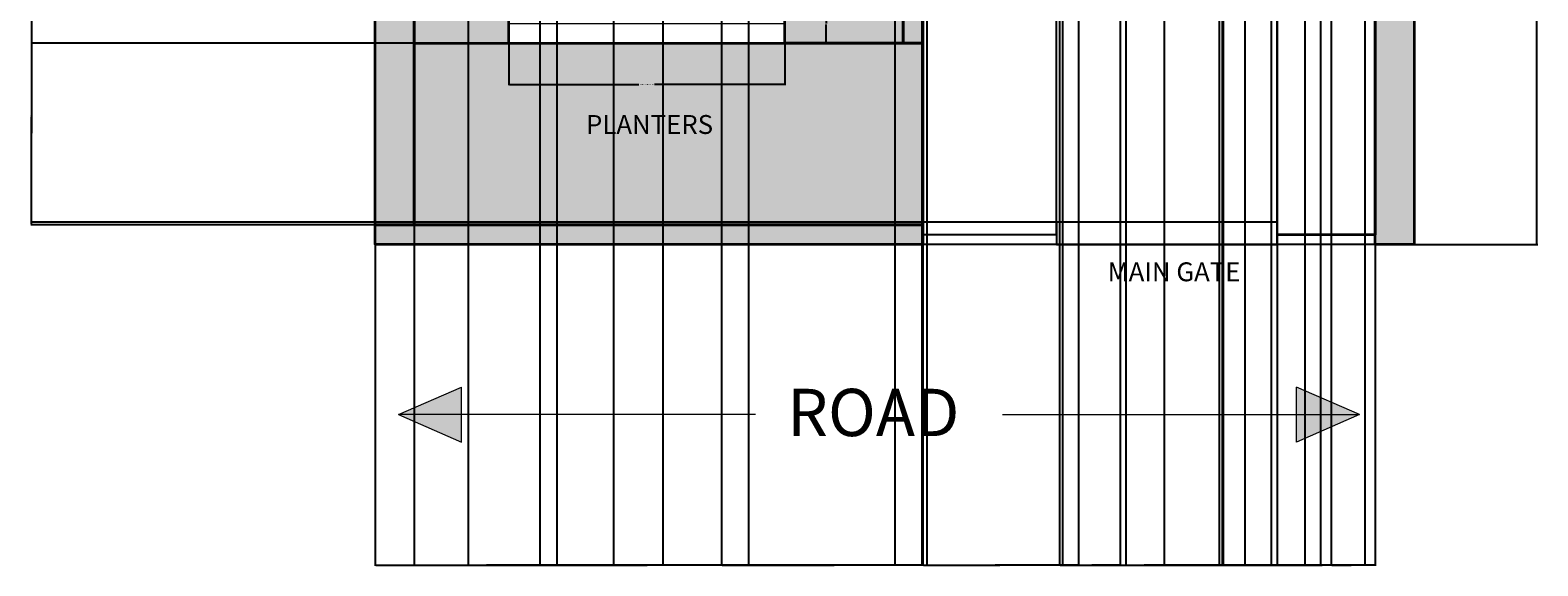
# Model space of a CAD drawing. Units: inches. Extents: x 2035 to 2384, y 1427 to 2020.
# Tile 1 of 7: x 2035 to 2383, y 1427 to 1551. Entities that reach past the tile are written whole.
import ezdxf

# ---------------------------------------------------------------- set-up
doc = ezdxf.new("R2010")
doc.units = ezdxf.units.IN
for name, color, linetype, lineweight in [('A-ANNO-DIMS', 2, 'Continuous', 18), ('A-ANNO-SYMB', 201, 'Continuous', 18), ('A-ANNO-TEXT', 201, 'Continuous', 18), ('A-SITE-GATE', 52, 'Continuous', 25), ('A-WALL-PATT', 140, 'Continuous', 13), ('C-PROP', 7, 'Continuous', 25), ('L-PLNT-PATT', 112, 'Continuous', 13), ('WALL', 140, 'Continuous', 35), ('WIN', 230, 'Continuous', 18)]:
    doc.layers.add(name, color=color, linetype=linetype, lineweight=lineweight)
doc.styles.get("Standard").update_dxf_attribs({"font": 'arial.ttf'})
doc.dimstyles.get("Standard").update_dxf_attribs({"dimtxt": 0.18, "dimasz": 0.18, "dimexe": 0.18, "dimexo": 0.0625, "dimgap": 0.09, "dimtad": 0, "dimtih": 1, "dimtoh": 1, "dimdec": 4, "dimzin": 0, "dimdsep": 46, "dimtxsty": 'Standard', "dimcen": 0.09, "dimadec": 0, "dimazin": 0, "dimtfac": 1, "dimtdec": 4, "dimtofl": 0, "dimtmove": 0, "dimatfit": 3, "dimfxl": 1, "dimtolj": 1, "dimtzin": 0, "dimarcsym": 0})

# ---------------------------------------------------------------- blocks, each defined once
blk = doc.blocks.new('WIN-BEDROOM')
blk.add_line((0, 4.5), (63.76, 4.5))
blk.add_lwpolyline([(0, 9), (63.76, 9), (63.76, 0), (0, 0)], close=True)
blk = doc.blocks.new('*D14')
at = {"layer": 'A-ANNO-DIMS', "color": 0, "lineweight": -2, "transparency": 16777216}
for p, q in [((2145.62, 1547.82), (2145.62, 1538.14)), ((2209.38, 1547.82), (2209.38, 1538.14)), ((2145.8, 1538.32), (2175.7, 1538.32)), ((2209.2, 1538.32), (2179.29, 1538.32))]:
    blk.add_line(p, q, dxfattribs=at)
at = {"layer": 'A-ANNO-DIMS', "color": 0, "lineweight": 100, "transparency": 16777216}
for points in [[(2145.8, 1538.35), (2145.8, 1538.29), (2145.62, 1538.32)], [(2209.2, 1538.35), (2209.2, 1538.29), (2209.38, 1538.32)]]:
    blk.add_solid(points, dxfattribs=at)
at = {"layer": 'Defpoints', "color": 0, "lineweight": 100, "transparency": 16777216}
for p in [(2145.62, 1547.88), (2209.38, 1547.88), (2209.38, 1538.32)]:
    blk.add_point(p, dxfattribs=at)
at = {"layer": 'A-ANNO-DIMS', "color": 0, "transparency": 16777216, "insert": (2177.5, 1538.32), "char_height": 0.18, "attachment_point": 5}
blk.add_mtext('\\A1;BEDROOM WINDOW 64 TYP.', dxfattribs=at)
blk = doc.blocks.new('*D15')
at = {"layer": 'A-ANNO-DIMS', "color": 0, "lineweight": -2, "transparency": 16777216}
for p, q in [((2209.44, 1556.88), (2219.12, 1556.88)), ((2218.94, 1556.7), (2218.94, 1552.56)), ((2218.94, 1548.06), (2218.94, 1552.2)), ((2209.44, 1547.88), (2219.12, 1547.88))]:
    blk.add_line(p, q, dxfattribs=at)
at = {"layer": 'A-ANNO-DIMS', "color": 0, "lineweight": 100, "transparency": 16777216}
for points in [[(2218.91, 1556.7), (2218.97, 1556.7), (2218.94, 1556.88)], [(2218.91, 1548.06), (2218.97, 1548.06), (2218.94, 1547.88)]]:
    blk.add_solid(points, dxfattribs=at)
at = {"layer": 'Defpoints', "color": 0, "lineweight": 100, "transparency": 16777216}
for p in [(2209.38, 1556.88), (2218.94, 1556.88), (2209.38, 1547.88)]:
    blk.add_point(p, dxfattribs=at)
at = {"layer": 'A-ANNO-DIMS', "color": 0, "transparency": 16777216, "insert": (2218.94, 1552.38), "char_height": 0.18, "attachment_point": 5}
blk.add_mtext('\\A1;9 TYP.', dxfattribs=at)
blk = doc.blocks.new('*D23')
at = {"layer": 'A-ANNO-DIMS', "color": 0, "lineweight": -2, "transparency": 16777216}
for p, q in [((2354.82, 1981.38), (2383.33, 1981.38)), ((2383.15, 1981.2), (2383.15, 1741.56)), ((2383.15, 1501.56), (2383.15, 1741.2)), ((2354.82, 1501.38), (2383.33, 1501.38))]:
    blk.add_line(p, q, dxfattribs=at)
at = {"layer": 'A-ANNO-DIMS', "color": 0, "lineweight": 100, "transparency": 16777216}
for points in [[(2383.12, 1981.2), (2383.18, 1981.2), (2383.15, 1981.38)], [(2383.12, 1501.56), (2383.18, 1501.56), (2383.15, 1501.38)]]:
    blk.add_solid(points, dxfattribs=at)
at = {"layer": 'Defpoints', "color": 0, "lineweight": 100, "transparency": 16777216}
for p in [(2354.75, 1981.38), (2383.15, 1981.38), (2354.75, 1501.38)]:
    blk.add_point(p, dxfattribs=at)
at = {"layer": 'A-ANNO-DIMS', "color": 0, "transparency": 16777216, "insert": (2383.15, 1741.38), "char_height": 0.18, "attachment_point": 5}
blk.add_mtext('\\A1;480', dxfattribs=at)
blk = doc.blocks.new('*D24')
at = {"layer": 'A-ANNO-DIMS', "color": 0, "lineweight": -2, "transparency": 16777216}
for p, q in [((2114.75, 1501.32), (2114.75, 1427.17)), ((2241.25, 1501.32), (2241.25, 1427.17)), ((2114.93, 1427.35), (2177.62, 1427.35)), ((2241.07, 1427.35), (2178.39, 1427.35))]:
    blk.add_line(p, q, dxfattribs=at)
at = {"layer": 'A-ANNO-DIMS', "color": 0, "lineweight": 100, "transparency": 16777216}
for points in [[(2114.93, 1427.38), (2114.93, 1427.32), (2114.75, 1427.35)], [(2241.07, 1427.38), (2241.07, 1427.32), (2241.25, 1427.35)]]:
    blk.add_solid(points, dxfattribs=at)
at = {"layer": 'Defpoints', "color": 0, "lineweight": 100, "transparency": 16777216}
for p in [(2114.75, 1501.38), (2241.25, 1501.38), (2241.25, 1427.35)]:
    blk.add_point(p, dxfattribs=at)
at = {"layer": 'A-ANNO-DIMS', "color": 0, "transparency": 16777216, "insert": (2178, 1427.35), "char_height": 0.18, "attachment_point": 5}
blk.add_mtext('\\A1;126.5', dxfattribs=at)
blk = doc.blocks.new('*D25')
at = {"layer": 'A-ANNO-DIMS', "color": 0, "lineweight": -2, "transparency": 16777216}
for p, q in [((2241.25, 1503.69), (2241.25, 2009.96)), ((2241.43, 2009.78), (2256.26, 2009.78)), ((2272.01, 2009.78), (2257.18, 2009.78)), ((2272.19, 1503.69), (2272.19, 2009.96))]:
    blk.add_line(p, q, dxfattribs=at)
at = {"layer": 'A-ANNO-DIMS', "color": 0, "lineweight": 100, "transparency": 16777216}
for points in [[(2241.43, 2009.81), (2241.43, 2009.75), (2241.25, 2009.78)], [(2272.01, 2009.81), (2272.01, 2009.75), (2272.19, 2009.78)]]:
    blk.add_solid(points, dxfattribs=at)
at = {"layer": 'Defpoints', "color": 0, "lineweight": 100, "transparency": 16777216}
for p in [(2272.19, 2009.78), (2241.25, 1503.63), (2272.19, 1503.63)]:
    blk.add_point(p, dxfattribs=at)
at = {"layer": 'A-ANNO-DIMS', "color": 0, "transparency": 16777216, "insert": (2256.72, 2009.78), "char_height": 0.18, "attachment_point": 5}
blk.add_mtext('\\A1;30.935', dxfattribs=at)
blk = doc.blocks.new('*D26')
at = {"layer": 'A-ANNO-DIMS', "color": 0, "lineweight": -2, "transparency": 16777216}
for p, q in [((2272.19, 1506.56), (2272.19, 2009.96)), ((2272.37, 2009.78), (2297.26, 2009.78)), ((2322.93, 2009.78), (2298.04, 2009.78)), ((2323.11, 1506.56), (2323.11, 2009.96))]:
    blk.add_line(p, q, dxfattribs=at)
at = {"layer": 'A-ANNO-DIMS', "color": 0, "lineweight": 100, "transparency": 16777216}
for points in [[(2272.37, 2009.81), (2272.37, 2009.75), (2272.19, 2009.78)], [(2322.93, 2009.81), (2322.93, 2009.75), (2323.11, 2009.78)]]:
    blk.add_solid(points, dxfattribs=at)
at = {"layer": 'Defpoints', "color": 0, "lineweight": 100, "transparency": 16777216}
for p in [(2323.11, 2009.78), (2272.19, 1506.5), (2323.11, 1506.5)]:
    blk.add_point(p, dxfattribs=at)
at = {"layer": 'A-ANNO-DIMS', "color": 0, "transparency": 16777216, "insert": (2297.65, 2009.78), "char_height": 0.18, "attachment_point": 5}
blk.add_mtext('\\A1;50.92', dxfattribs=at)
blk = doc.blocks.new('*D27')
at = {"layer": 'A-ANNO-DIMS', "color": 0, "lineweight": -2, "transparency": 16777216}
for p, q in [((2123.69, 1547.88), (2035.17, 1547.88)), ((2035.35, 1547.7), (2035.35, 1527.06)), ((2035.35, 1506.06), (2035.35, 1526.7)), ((2123.69, 1505.88), (2035.17, 1505.88))]:
    blk.add_line(p, q, dxfattribs=at)
at = {"layer": 'A-ANNO-DIMS', "color": 0, "lineweight": 100, "transparency": 16777216}
for points in [[(2035.32, 1547.7), (2035.38, 1547.7), (2035.35, 1547.88)], [(2035.32, 1506.06), (2035.38, 1506.06), (2035.35, 1505.88)]]:
    blk.add_solid(points, dxfattribs=at)
at = {"layer": 'Defpoints', "color": 0, "lineweight": 100, "transparency": 16777216}
for p in [(2035.35, 1547.88), (2123.75, 1547.88), (2123.75, 1505.88)]:
    blk.add_point(p, dxfattribs=at)
at = {"layer": 'A-ANNO-DIMS', "color": 0, "transparency": 16777216, "insert": (2035.35, 1526.88), "char_height": 0.18, "attachment_point": 5}
blk.add_mtext('\\A1;42', dxfattribs=at)
blk = doc.blocks.new('*D28')
at = {"layer": 'A-ANNO-DIMS', "color": 0, "lineweight": -2, "transparency": 16777216}
for p, q in [((2345.69, 1555.63), (2035.17, 1555.63)), ((2035.35, 1555.45), (2035.35, 1531.25)), ((2035.35, 1506.68), (2035.35, 1530.88)), ((2323.05, 1506.5), (2035.17, 1506.5))]:
    blk.add_line(p, q, dxfattribs=at)
at = {"layer": 'A-ANNO-DIMS', "color": 0, "lineweight": 100, "transparency": 16777216}
for points in [[(2035.32, 1555.45), (2035.38, 1555.45), (2035.35, 1555.63)], [(2035.32, 1506.68), (2035.38, 1506.68), (2035.35, 1506.5)]]:
    blk.add_solid(points, dxfattribs=at)
at = {"layer": 'Defpoints', "color": 0, "lineweight": 100, "transparency": 16777216}
for p in [(2035.35, 1555.63), (2345.75, 1555.63), (2323.11, 1506.5)]:
    blk.add_point(p, dxfattribs=at)
at = {"layer": 'A-ANNO-DIMS', "color": 0, "transparency": 16777216, "insert": (2035.35, 1531.06), "char_height": 0.18, "attachment_point": 5}
blk.add_mtext('\\A1;49.14', dxfattribs=at)
blk = doc.blocks.new('*D31')
at = {"layer": 'A-ANNO-DIMS', "color": 0, "lineweight": -2, "transparency": 16777216}
for p, q in [((2241.25, 1555.57), (2241.25, 1427.17)), ((2277.25, 1555.57), (2277.25, 1427.17)), ((2241.43, 1427.35), (2259.03, 1427.35)), ((2277.07, 1427.35), (2259.47, 1427.35))]:
    blk.add_line(p, q, dxfattribs=at)
at = {"layer": 'A-ANNO-DIMS', "color": 0, "lineweight": 100, "transparency": 16777216}
for points in [[(2241.43, 1427.38), (2241.43, 1427.32), (2241.25, 1427.35)], [(2277.07, 1427.38), (2277.07, 1427.32), (2277.25, 1427.35)]]:
    blk.add_solid(points, dxfattribs=at)
at = {"layer": 'Defpoints', "color": 0, "lineweight": 100, "transparency": 16777216}
for p in [(2241.25, 1555.63), (2277.25, 1555.63), (2277.25, 1427.35)]:
    blk.add_point(p, dxfattribs=at)
at = {"layer": 'A-ANNO-DIMS', "color": 0, "transparency": 16777216, "insert": (2259.25, 1427.35), "char_height": 0.18, "attachment_point": 5}
blk.add_mtext('\\A1;36', dxfattribs=at)
blk = doc.blocks.new('*D32')
at = {"layer": 'A-ANNO-DIMS', "color": 0, "lineweight": -2, "transparency": 16777216}
for p, q in [((2277.25, 1555.57), (2277.25, 1427.17)), ((2309.75, 1555.57), (2309.75, 1427.17)), ((2277.43, 1427.35), (2293.18, 1427.35)), ((2309.57, 1427.35), (2293.83, 1427.35))]:
    blk.add_line(p, q, dxfattribs=at)
at = {"layer": 'A-ANNO-DIMS', "color": 0, "lineweight": 100, "transparency": 16777216}
for points in [[(2277.43, 1427.38), (2277.43, 1427.32), (2277.25, 1427.35)], [(2309.57, 1427.38), (2309.57, 1427.32), (2309.75, 1427.35)]]:
    blk.add_solid(points, dxfattribs=at)
at = {"layer": 'Defpoints', "color": 0, "lineweight": 100, "transparency": 16777216}
for p in [(2277.25, 1555.63), (2309.75, 1555.63), (2309.75, 1427.35)]:
    blk.add_point(p, dxfattribs=at)
at = {"layer": 'A-ANNO-DIMS', "color": 0, "transparency": 16777216, "insert": (2293.5, 1427.35), "char_height": 0.18, "attachment_point": 5}
blk.add_mtext('\\A1;32.5', dxfattribs=at)
blk = doc.blocks.new('*D34')
at = {"layer": 'A-ANNO-DIMS', "color": 0, "lineweight": -2, "transparency": 16777216}
for p, q in [((2194.77, 1680.82), (2194.77, 1427.17)), ((2234.77, 1680.82), (2234.77, 1427.17)), ((2194.95, 1427.35), (2214.55, 1427.35)), ((2234.59, 1427.35), (2214.99, 1427.35))]:
    blk.add_line(p, q, dxfattribs=at)
at = {"layer": 'A-ANNO-DIMS', "color": 0, "lineweight": 100, "transparency": 16777216}
for points in [[(2194.95, 1427.38), (2194.95, 1427.32), (2194.77, 1427.35)], [(2234.59, 1427.38), (2234.59, 1427.32), (2234.77, 1427.35)]]:
    blk.add_solid(points, dxfattribs=at)
at = {"layer": 'Defpoints', "color": 0, "lineweight": 100, "transparency": 16777216}
for p in [(2194.77, 1680.88), (2234.77, 1680.88), (2234.77, 1427.35)]:
    blk.add_point(p, dxfattribs=at)
at = {"layer": 'A-ANNO-DIMS', "color": 0, "transparency": 16777216, "insert": (2214.77, 1427.35), "char_height": 0.18, "attachment_point": 5}
blk.add_mtext('\\A1;40', dxfattribs=at)
blk = doc.blocks.new('*D35')
at = {"layer": 'A-ANNO-DIMS', "color": 0, "lineweight": -2, "transparency": 16777216}
for p, q in [((2242.18, 1680.82), (2242.18, 1427.17)), ((2272.85, 1680.82), (2272.85, 1427.17)), ((2242.36, 1427.35), (2257.05, 1427.35)), ((2272.67, 1427.35), (2257.98, 1427.35))]:
    blk.add_line(p, q, dxfattribs=at)
at = {"layer": 'A-ANNO-DIMS', "color": 0, "lineweight": 100, "transparency": 16777216}
for points in [[(2242.36, 1427.38), (2242.36, 1427.32), (2242.18, 1427.35)], [(2272.67, 1427.38), (2272.67, 1427.32), (2272.85, 1427.35)]]:
    blk.add_solid(points, dxfattribs=at)
at = {"layer": 'Defpoints', "color": 0, "lineweight": 100, "transparency": 16777216}
for p in [(2242.18, 1680.88), (2272.85, 1680.88), (2272.85, 1427.35)]:
    blk.add_point(p, dxfattribs=at)
at = {"layer": 'A-ANNO-DIMS', "color": 0, "transparency": 16777216, "insert": (2257.52, 1427.35), "char_height": 0.18, "attachment_point": 5}
blk.add_mtext('\\A1;30.676', dxfattribs=at)
blk = doc.blocks.new('*D36')
at = {"layer": 'A-ANNO-DIMS', "color": 0, "lineweight": -2, "transparency": 16777216}
for p, q in [((2286.88, 1680.82), (2286.88, 1427.17)), ((2329.51, 1680.82), (2329.51, 1427.17)), ((2287.06, 1427.35), (2307.8, 1427.35)), ((2329.33, 1427.35), (2308.59, 1427.35))]:
    blk.add_line(p, q, dxfattribs=at)
at = {"layer": 'A-ANNO-DIMS', "color": 0, "lineweight": 100, "transparency": 16777216}
for points in [[(2287.06, 1427.38), (2287.06, 1427.32), (2286.88, 1427.35)], [(2329.33, 1427.38), (2329.33, 1427.32), (2329.51, 1427.35)]]:
    blk.add_solid(points, dxfattribs=at)
at = {"layer": 'Defpoints', "color": 0, "lineweight": 100, "transparency": 16777216}
for p in [(2286.88, 1680.88), (2329.51, 1680.88), (2329.51, 1427.35)]:
    blk.add_point(p, dxfattribs=at)
at = {"layer": 'A-ANNO-DIMS', "color": 0, "transparency": 16777216, "insert": (2308.2, 1427.35), "char_height": 0.18, "attachment_point": 5}
blk.add_mtext('\\A1;42.63', dxfattribs=at)
blk = doc.blocks.new('*D37')
at = {"layer": 'A-ANNO-DIMS', "color": 0, "lineweight": -2, "transparency": 16777216}
for p, q in [((2152.83, 1680.82), (2152.83, 1427.17)), ((2181.2, 1680.82), (2181.2, 1427.17)), ((2153.01, 1427.35), (2166.62, 1427.35)), ((2181.02, 1427.35), (2167.41, 1427.35))]:
    blk.add_line(p, q, dxfattribs=at)
at = {"layer": 'A-ANNO-DIMS', "color": 0, "lineweight": 100, "transparency": 16777216}
for points in [[(2153.01, 1427.38), (2153.01, 1427.32), (2152.83, 1427.35)], [(2181.02, 1427.38), (2181.02, 1427.32), (2181.2, 1427.35)]]:
    blk.add_solid(points, dxfattribs=at)
at = {"layer": 'Defpoints', "color": 0, "lineweight": 100, "transparency": 16777216}
for p in [(2152.83, 1680.88), (2181.2, 1680.88), (2181.2, 1427.35)]:
    blk.add_point(p, dxfattribs=at)
at = {"layer": 'A-ANNO-DIMS', "color": 0, "transparency": 16777216, "insert": (2167.02, 1427.35), "char_height": 0.18, "attachment_point": 5}
blk.add_mtext('\\A1;28.37', dxfattribs=at)
blk = doc.blocks.new('*D39')
at = {"layer": 'A-ANNO-DIMS', "color": 0, "lineweight": -2, "transparency": 16777216}
for p, q in [((2136.25, 1759.32), (2136.25, 1427.17)), ((2169.78, 1759.32), (2169.78, 1427.17)), ((2136.43, 1427.35), (2152.62, 1427.35)), ((2169.6, 1427.35), (2153.41, 1427.35))]:
    blk.add_line(p, q, dxfattribs=at)
at = {"layer": 'A-ANNO-DIMS', "color": 0, "lineweight": 100, "transparency": 16777216}
for points in [[(2136.43, 1427.38), (2136.43, 1427.32), (2136.25, 1427.35)], [(2169.6, 1427.38), (2169.6, 1427.32), (2169.78, 1427.35)]]:
    blk.add_solid(points, dxfattribs=at)
at = {"layer": 'Defpoints', "color": 0, "lineweight": 100, "transparency": 16777216}
for p in [(2136.25, 1759.38), (2169.78, 1759.38), (2169.78, 1427.35)]:
    blk.add_point(p, dxfattribs=at)
at = {"layer": 'A-ANNO-DIMS', "color": 0, "transparency": 16777216, "insert": (2153.02, 1427.35), "char_height": 0.18, "attachment_point": 5}
blk.add_mtext('\\A1;33.52', dxfattribs=at)
blk = doc.blocks.new('*D40')
at = {"layer": 'A-ANNO-DIMS', "color": 0, "lineweight": -2, "transparency": 16777216}
for p, q in [((2201.01, 1835.82), (2201.01, 1427.17)), ((2241.01, 1835.82), (2241.01, 1427.17)), ((2201.19, 1427.35), (2220.79, 1427.35)), ((2240.83, 1427.35), (2221.24, 1427.35))]:
    blk.add_line(p, q, dxfattribs=at)
at = {"layer": 'A-ANNO-DIMS', "color": 0, "lineweight": 100, "transparency": 16777216}
for points in [[(2201.19, 1427.38), (2201.19, 1427.32), (2201.01, 1427.35)], [(2240.83, 1427.38), (2240.83, 1427.32), (2241.01, 1427.35)]]:
    blk.add_solid(points, dxfattribs=at)
at = {"layer": 'Defpoints', "color": 0, "lineweight": 100, "transparency": 16777216}
for p in [(2201.01, 1835.88), (2241.01, 1835.88), (2241.01, 1427.35)]:
    blk.add_point(p, dxfattribs=at)
at = {"layer": 'A-ANNO-DIMS', "color": 0, "transparency": 16777216, "insert": (2221.01, 1427.35), "char_height": 0.18, "attachment_point": 5}
blk.add_mtext('\\A1;40', dxfattribs=at)
blk = doc.blocks.new('*D41')
at = {"layer": 'A-ANNO-DIMS', "color": 0, "lineweight": -2, "transparency": 16777216}
for p, q in [((2273.51, 1840.32), (2273.51, 1427.17)), ((2310.46, 1840.32), (2310.46, 1427.17)), ((2273.69, 1427.35), (2291.59, 1427.35)), ((2310.28, 1427.35), (2292.38, 1427.35))]:
    blk.add_line(p, q, dxfattribs=at)
at = {"layer": 'A-ANNO-DIMS', "color": 0, "lineweight": 100, "transparency": 16777216}
for points in [[(2273.69, 1427.38), (2273.69, 1427.32), (2273.51, 1427.35)], [(2310.28, 1427.38), (2310.28, 1427.32), (2310.46, 1427.35)]]:
    blk.add_solid(points, dxfattribs=at)
at = {"layer": 'Defpoints', "color": 0, "lineweight": 100, "transparency": 16777216}
for p in [(2273.51, 1840.38), (2310.46, 1840.38), (2310.46, 1427.35)]:
    blk.add_point(p, dxfattribs=at)
at = {"layer": 'A-ANNO-DIMS', "color": 0, "transparency": 16777216, "insert": (2291.98, 1427.35), "char_height": 0.18, "attachment_point": 5}
blk.add_mtext('\\A1;36.95', dxfattribs=at)
blk = doc.blocks.new('*D42')
at = {"layer": 'A-ANNO-DIMS', "color": 0, "lineweight": -2, "transparency": 16777216}
for p, q in [((2297.05, 1925.82), (2297.05, 1427.17)), ((2333.11, 1925.82), (2333.11, 1427.17)), ((2297.23, 1427.35), (2314.69, 1427.35)), ((2332.93, 1427.35), (2315.47, 1427.35))]:
    blk.add_line(p, q, dxfattribs=at)
at = {"layer": 'A-ANNO-DIMS', "color": 0, "lineweight": 100, "transparency": 16777216}
for points in [[(2297.23, 1427.38), (2297.23, 1427.32), (2297.05, 1427.35)], [(2332.93, 1427.38), (2332.93, 1427.32), (2333.11, 1427.35)]]:
    blk.add_solid(points, dxfattribs=at)
at = {"layer": 'Defpoints', "color": 0, "lineweight": 100, "transparency": 16777216}
for p in [(2297.05, 1925.88), (2333.11, 1925.88), (2333.11, 1427.35)]:
    blk.add_point(p, dxfattribs=at)
at = {"layer": 'A-ANNO-DIMS', "color": 0, "transparency": 16777216, "insert": (2315.08, 1427.35), "char_height": 0.18, "attachment_point": 5}
blk.add_mtext('\\A1;36.06', dxfattribs=at)
blk = doc.blocks.new('*D45')
at = {"layer": 'A-ANNO-DIMS', "color": 0, "lineweight": -2, "transparency": 16777216}
for p, q in [((2321.75, 1840.32), (2321.75, 1427.17)), ((2345.75, 1840.32), (2345.75, 1427.17)), ((2321.93, 1427.35), (2333.53, 1427.35)), ((2345.57, 1427.35), (2333.97, 1427.35))]:
    blk.add_line(p, q, dxfattribs=at)
at = {"layer": 'A-ANNO-DIMS', "color": 0, "lineweight": 100, "transparency": 16777216}
for points in [[(2321.93, 1427.38), (2321.93, 1427.32), (2321.75, 1427.35)], [(2345.57, 1427.38), (2345.57, 1427.32), (2345.75, 1427.35)]]:
    blk.add_solid(points, dxfattribs=at)
at = {"layer": 'Defpoints', "color": 0, "lineweight": 100, "transparency": 16777216}
for p in [(2321.75, 1840.38), (2345.75, 1840.38), (2345.75, 1427.35)]:
    blk.add_point(p, dxfattribs=at)
at = {"layer": 'A-ANNO-DIMS', "color": 0, "transparency": 16777216, "insert": (2333.75, 1427.35), "char_height": 0.18, "attachment_point": 5}
blk.add_mtext('\\A1;24', dxfattribs=at)
blk = doc.blocks.new('*D46')
at = {"layer": 'A-ANNO-DIMS', "color": 0, "lineweight": -2, "transparency": 16777216}
for p, q in [((2288.19, 1905.68), (2288.19, 1427.17)), ((2315.66, 1905.68), (2315.66, 1427.17)), ((2288.37, 1427.35), (2301.53, 1427.35)), ((2315.48, 1427.35), (2302.32, 1427.35))]:
    blk.add_line(p, q, dxfattribs=at)
at = {"layer": 'A-ANNO-DIMS', "color": 0, "lineweight": 100, "transparency": 16777216}
for points in [[(2288.37, 1427.38), (2288.37, 1427.32), (2288.19, 1427.35)], [(2315.48, 1427.38), (2315.48, 1427.32), (2315.66, 1427.35)]]:
    blk.add_solid(points, dxfattribs=at)
at = {"layer": 'Defpoints', "color": 0, "lineweight": 100, "transparency": 16777216}
for p in [(2288.19, 1905.75), (2315.66, 1905.75), (2315.66, 1427.35)]:
    blk.add_point(p, dxfattribs=at)
at = {"layer": 'A-ANNO-DIMS', "color": 0, "transparency": 16777216, "insert": (2301.92, 1427.35), "char_height": 0.18, "attachment_point": 5}
blk.add_mtext('\\A1;27.47', dxfattribs=at)
blk = doc.blocks.new('*D48')
at = {"layer": 'A-ANNO-DIMS', "color": 0, "lineweight": -2, "transparency": 16777216}
for p, q in [((2323.12, 1858.3), (2323.12, 1427.17)), ((2343.42, 1858.3), (2343.42, 1427.17)), ((2323.3, 1427.35), (2332.81, 1427.35)), ((2343.24, 1427.35), (2333.74, 1427.35))]:
    blk.add_line(p, q, dxfattribs=at)
at = {"layer": 'A-ANNO-DIMS', "color": 0, "lineweight": 100, "transparency": 16777216}
for points in [[(2323.3, 1427.38), (2323.3, 1427.32), (2323.12, 1427.35)], [(2343.24, 1427.38), (2343.24, 1427.32), (2343.42, 1427.35)]]:
    blk.add_solid(points, dxfattribs=at)
at = {"layer": 'Defpoints', "color": 0, "lineweight": 100, "transparency": 16777216}
for p in [(2323.12, 1858.36), (2343.42, 1858.36), (2343.42, 1427.35)]:
    blk.add_point(p, dxfattribs=at)
at = {"layer": 'A-ANNO-DIMS', "color": 0, "transparency": 16777216, "insert": (2333.27, 1427.35), "char_height": 0.18, "attachment_point": 5}
blk.add_mtext('\\A1;20.302', dxfattribs=at)
blk = doc.blocks.new('*D50')
at = {"layer": 'A-ANNO-DIMS', "color": 0, "lineweight": -2, "transparency": 16777216}
for p, q in [((2156.75, 1782.6), (2156.75, 1427.17)), ((2123.75, 1772.1), (2123.75, 1427.17)), ((2123.93, 1427.35), (2140.03, 1427.35)), ((2156.57, 1427.35), (2140.47, 1427.35))]:
    blk.add_line(p, q, dxfattribs=at)
at = {"layer": 'A-ANNO-DIMS', "color": 0, "lineweight": 100, "transparency": 16777216}
for points in [[(2123.93, 1427.38), (2123.93, 1427.32), (2123.75, 1427.35)], [(2156.57, 1427.38), (2156.57, 1427.32), (2156.75, 1427.35)]]:
    blk.add_solid(points, dxfattribs=at)
at = {"layer": 'Defpoints', "color": 0, "lineweight": 100, "transparency": 16777216}
for p in [(2156.75, 1782.66), (2123.75, 1772.16), (2156.75, 1427.35)]:
    blk.add_point(p, dxfattribs=at)
at = {"layer": 'A-ANNO-DIMS', "color": 0, "transparency": 16777216, "insert": (2140.25, 1427.35), "char_height": 0.18, "attachment_point": 5}
blk.add_mtext('\\A1;33', dxfattribs=at)
blk = doc.blocks.new('*D57')
at = {"layer": 'A-ANNO-DIMS', "color": 0, "lineweight": -2, "transparency": 16777216}
for p, q in [((2310.65, 1726.38), (2310.65, 1427.17)), ((2335.58, 1723.97), (2335.58, 1427.17)), ((2310.83, 1427.35), (2322.65, 1427.35)), ((2335.4, 1427.35), (2323.58, 1427.35))]:
    blk.add_line(p, q, dxfattribs=at)
at = {"layer": 'A-ANNO-DIMS', "color": 0, "lineweight": 100, "transparency": 16777216}
for points in [[(2310.83, 1427.38), (2310.83, 1427.32), (2310.65, 1427.35)], [(2335.4, 1427.38), (2335.4, 1427.32), (2335.58, 1427.35)]]:
    blk.add_solid(points, dxfattribs=at)
at = {"layer": 'Defpoints', "color": 0, "lineweight": 100, "transparency": 16777216}
for p in [(2310.65, 1726.45), (2335.58, 1724.03), (2335.58, 1427.35)]:
    blk.add_point(p, dxfattribs=at)
at = {"layer": 'A-ANNO-DIMS', "color": 0, "transparency": 16777216, "insert": (2323.12, 1427.35), "char_height": 0.18, "attachment_point": 5}
blk.add_mtext('\\A1;24.924', dxfattribs=at)
blk = doc.blocks.new('*D64')
at = {"layer": 'A-ANNO-DIMS', "color": 0, "lineweight": -2, "transparency": 16777216}
for p, q in [((2335.58, 1723.97), (2335.58, 1427.17)), ((2345.75, 1685.32), (2345.75, 1427.17)), ((2335.76, 1427.35), (2340.21, 1427.35)), ((2345.57, 1427.35), (2341.12, 1427.35))]:
    blk.add_line(p, q, dxfattribs=at)
at = {"layer": 'A-ANNO-DIMS', "color": 0, "lineweight": 100, "transparency": 16777216}
for points in [[(2335.76, 1427.38), (2335.76, 1427.32), (2335.58, 1427.35)], [(2345.57, 1427.38), (2345.57, 1427.32), (2345.75, 1427.35)]]:
    blk.add_solid(points, dxfattribs=at)
at = {"layer": 'Defpoints', "color": 0, "lineweight": 100, "transparency": 16777216}
for p in [(2335.58, 1724.03), (2345.75, 1685.38), (2345.75, 1427.35)]:
    blk.add_point(p, dxfattribs=at)
at = {"layer": 'A-ANNO-DIMS', "color": 0, "transparency": 16777216, "insert": (2340.67, 1427.35), "char_height": 0.18, "attachment_point": 5}
blk.add_mtext('\\A1;10.174', dxfattribs=at)
blk = doc.blocks.new('*D67')
at = {"layer": 'A-ANNO-DIMS', "color": 0, "lineweight": -2, "transparency": 16777216}
for p, q in [((2272.85, 1680.82), (2272.85, 1427.17)), ((2286.88, 1680.82), (2286.88, 1427.17)), ((2273.03, 1427.35), (2279.41, 1427.35)), ((2286.7, 1427.35), (2280.32, 1427.35))]:
    blk.add_line(p, q, dxfattribs=at)
at = {"layer": 'A-ANNO-DIMS', "color": 0, "lineweight": 100, "transparency": 16777216}
for points in [[(2273.03, 1427.38), (2273.03, 1427.32), (2272.85, 1427.35)], [(2286.7, 1427.38), (2286.7, 1427.32), (2286.88, 1427.35)]]:
    blk.add_solid(points, dxfattribs=at)
at = {"layer": 'Defpoints', "color": 0, "lineweight": 100, "transparency": 16777216}
for p in [(2272.85, 1680.88), (2286.88, 1680.88), (2286.88, 1427.35)]:
    blk.add_point(p, dxfattribs=at)
at = {"layer": 'A-ANNO-DIMS', "color": 0, "transparency": 16777216, "insert": (2279.87, 1427.35), "char_height": 0.18, "attachment_point": 5}
blk.add_mtext('\\A1;14.025', dxfattribs=at)

msp = doc.modelspace()

# ---------------------------------------------------------------- hatches: boundary and pattern name
at = {"layer": 'A-ANNO-SYMB'}
h = msp.add_hatch(color=256, dxfattribs=at)
h.dxf.hatch_style = 1
h.paths.add_polyline_path([(2134.692, 1468.4496), (2120.1051, 1462.0989), (2134.692, 1462.0989)])
h.paths.add_polyline_path([(2134.692, 1462.0989), (2120.1051, 1462.0989), (2134.692, 1455.7483)])
h = msp.add_hatch(color=256, dxfattribs=at)
h.dxf.hatch_style = 1
h.paths.add_polyline_path([(2342.172, 1462.0989), (2327.5851, 1468.4496), (2327.5851, 1462.0989)])
h.paths.add_polyline_path([(2342.172, 1462.0989), (2327.5851, 1462.0989), (2327.5851, 1455.7483)])
at = {"layer": 'A-WALL-PATT'}
h = msp.add_hatch(color=256, dxfattribs=at)
h.dxf.hatch_style = 1
h.paths.add_polyline_path([(2145.6215, 1981.3816), (2123.7529, 1981.3816), (2123.7529, 1972.3816), (2145.6215, 1972.3816)])
h.paths.add_polyline_path([(2354.7529, 1981.3816), (2209.3767, 1981.3816), (2209.3767, 1972.3816), (2354.7529, 1972.3816)])
h.paths.add_polyline_path([(2123.7529, 1981.3816), (2114.7529, 1981.3816), (2114.7529, 1505.8816), (2123.7529, 1505.8816)])
h.paths.add_polyline_path([(2248.2529, 1928.1316), (2243.7529, 1928.1316), (2243.7529, 1840.3816), (2248.2529, 1840.3816)])
h.paths.add_polyline_path([(2297.0514, 1930.3816), (2284.6994, 1930.3816), (2284.6994, 1925.8816), (2297.0514, 1925.8816)])
h.paths.add_polyline_path([(2345.7529, 1930.3816), (2333.1098, 1930.3816), (2333.1098, 1925.8816), (2345.7529, 1925.8816)])
h.paths.add_polyline_path([(2354.7529, 1972.3816), (2345.7529, 1972.3816), (2345.7529, 1501.3816), (2354.7529, 1501.3816)])
h.paths.add_polyline_path([(2188.2529, 1835.8816), (2183.7529, 1835.8816), (2183.7529, 1831.3677), (2184.207, 1831.3677), (2188.2529, 1831.3677)])
h.paths.add_polyline_path([(2188.2529, 1804.3949), (2184.207, 1804.3949), (2183.7529, 1804.3949), (2183.7529, 1685.3816), (2188.2529, 1685.3816)])
h.paths.add_polyline_path([(2273.5087, 1840.3816), (2241.0146, 1840.3816), (2241.0146, 1835.8816), (2273.5087, 1835.8816)])
h.paths.add_polyline_path([(2345.7529, 1840.3816), (2310.4577, 1840.3816), (2310.4577, 1835.8816), (2345.7529, 1835.8816)])
h.paths.add_polyline_path([(2161.9064, 1524.4315), (2196.2972, 1524.4315), (2196.2972, 1533.4306), (2161.9064, 1533.4306)], flags=9)
h.paths.add_polyline_path([(2279.3058, 1589.7515), (2308.9483, 1589.7515), (2308.9483, 1598.7506), (2279.3058, 1598.7506)], flags=9)
h.paths.add_polyline_path([(2242.9684, 1662.1655), (2279.0513, 1662.1655), (2279.0513, 1671.1647), (2242.9684, 1671.1647)], flags=9)
h.paths.add_polyline_path([(2154.6483, 1622.8242), (2195.1309, 1622.8242), (2195.1309, 1639.1195), (2154.6483, 1639.1195)], flags=9)
h.paths.add_polyline_path([(2138.8708, 1715.378), (2162.5199, 1715.378), (2162.5199, 1731.6734), (2138.8708, 1731.6734)], flags=9)
h.paths.add_polyline_path([(2135.5598, 1791.707), (2165.1993, 1791.707), (2165.1993, 1808.0024), (2135.5598, 1808.0024)], flags=9)
h.paths.add_polyline_path([(2245.1071, 1740.4502), (2279.0303, 1740.4502), (2279.0303, 1756.7455), (2245.1071, 1756.7455)], flags=9)
h.paths.add_polyline_path([(2284.7312, 1866.5552), (2313.6916, 1866.5552), (2313.6916, 1890.2034), (2284.7312, 1890.2034)], flags=9)
h.paths.add_polyline_path([(2139.9071, 1874.6496), (2173.8303, 1874.6496), (2173.8303, 1890.9449), (2139.9071, 1890.9449)], flags=9)
h = msp.add_hatch(color=256, dxfattribs=at)
h.dxf.hatch_style = 1
h.paths.add_polyline_path([(2236.7529, 1556.8816), (2209.3767, 1556.8816), (2209.3767, 1547.8816), (2236.7529, 1547.8816)])
h.paths.add_polyline_path([(2241.2529, 1680.8816), (2236.7529, 1680.8816), (2236.7529, 1547.8816), (2241.2529, 1547.8816)])
h.paths.add_polyline_path([(2241.2529, 1505.8816), (2114.7529, 1505.8816), (2114.7529, 1501.3816), (2241.2529, 1501.3816)])
h.paths.add_polyline_path([(2242.179, 1683.1823), (2242.179, 1685.3816), (2234.769, 1685.3816), (2234.769, 1680.8816), (2242.179, 1680.8816)])
h.paths.add_polyline_path([(2286.8795, 1685.3816), (2272.8549, 1685.3816), (2272.8549, 1683.1823), (2272.8549, 1680.8816), (2286.8795, 1680.8816)])
h.paths.add_polyline_path([(2345.7529, 1685.3816), (2329.513, 1685.3816), (2329.513, 1680.8816), (2345.7529, 1680.8816)])
h.paths.add_polyline_path([(2279.3058, 1589.7515), (2308.9483, 1589.7515), (2308.9483, 1598.7506), (2279.3058, 1598.7506)], flags=9)
h.paths.add_polyline_path([(2242.9684, 1662.1655), (2279.0513, 1662.1655), (2279.0513, 1671.1647), (2242.9684, 1671.1647)], flags=9)
h.paths.add_polyline_path([(2154.6483, 1622.8242), (2195.1309, 1622.8242), (2195.1309, 1639.1195), (2154.6483, 1639.1195)], flags=9)
h.paths.add_polyline_path([(2138.8708, 1715.378), (2162.5199, 1715.378), (2162.5199, 1731.6734), (2138.8708, 1731.6734)], flags=9)
h.paths.add_polyline_path([(2135.5598, 1791.707), (2165.1993, 1791.707), (2165.1993, 1808.0024), (2135.5598, 1808.0024)], flags=9)
h.paths.add_polyline_path([(2245.1071, 1740.4502), (2279.0303, 1740.4502), (2279.0303, 1756.7455), (2245.1071, 1756.7455)], flags=9)
h.paths.add_polyline_path([(2284.7312, 1866.5552), (2313.6916, 1866.5552), (2313.6916, 1890.2034), (2284.7312, 1890.2034)], flags=9)
h.paths.add_polyline_path([(2284.6985, 1943.1527), (2309.7208, 1943.1527), (2309.7208, 1959.448), (2284.6985, 1959.448)], flags=9)
h.paths.add_polyline_path([(2139.9071, 1874.6496), (2173.8303, 1874.6496), (2173.8303, 1890.9449), (2139.9071, 1890.9449)], flags=9)
h = msp.add_hatch(color=256, dxfattribs=at)
h.dxf.hatch_style = 1
h.paths.add_polyline_path([(2201.0146, 1840.3816), (2123.7529, 1840.3816), (2123.7529, 1835.8816), (2201.0146, 1835.8816)])
h.paths.add_polyline_path([(2136.2543, 1763.8816), (2123.7529, 1763.8816), (2123.7529, 1759.3816), (2136.2543, 1759.3816)])
h.paths.add_polyline_path([(2183.7529, 1763.8816), (2169.7769, 1763.8816), (2169.7769, 1759.3816), (2183.7529, 1759.3816)])
h.paths.add_polyline_path([(2152.8338, 1685.1369), (2152.8338, 1685.3816), (2123.7529, 1685.3816), (2123.7529, 1680.8816), (2152.8338, 1680.8816)])
h.paths.add_polyline_path([(2194.769, 1685.3816), (2181.2028, 1685.3816), (2181.2028, 1685.1369), (2181.2028, 1680.8816), (2194.769, 1680.8816)])
h.paths.add_polyline_path([(2145.6215, 1556.8816), (2123.7529, 1556.8816), (2123.7529, 1547.8816), (2145.6215, 1547.8816)])
h.paths.add_polyline_path([(2161.9064, 1524.4315), (2196.2972, 1524.4315), (2196.2972, 1533.4306), (2161.9064, 1533.4306)], flags=9)
h.paths.add_polyline_path([(2279.3058, 1589.7515), (2308.9483, 1589.7515), (2308.9483, 1598.7506), (2279.3058, 1598.7506)], flags=9)
h.paths.add_polyline_path([(2242.9684, 1662.1655), (2279.0513, 1662.1655), (2279.0513, 1671.1647), (2242.9684, 1671.1647)], flags=9)
h.paths.add_polyline_path([(2154.6483, 1622.8242), (2195.1309, 1622.8242), (2195.1309, 1639.1195), (2154.6483, 1639.1195)], flags=9)
h.paths.add_polyline_path([(2138.8708, 1715.378), (2162.5199, 1715.378), (2162.5199, 1731.6734), (2138.8708, 1731.6734)], flags=9)
h.paths.add_polyline_path([(2135.5598, 1791.707), (2165.1993, 1791.707), (2165.1993, 1808.0024), (2135.5598, 1808.0024)], flags=9)
h.paths.add_polyline_path([(2245.1071, 1740.4502), (2279.0303, 1740.4502), (2279.0303, 1756.7455), (2245.1071, 1756.7455)], flags=9)
h.paths.add_polyline_path([(2284.7312, 1866.5552), (2313.6916, 1866.5552), (2313.6916, 1890.2034), (2284.7312, 1890.2034)], flags=9)
h.paths.add_polyline_path([(2284.6985, 1943.1527), (2309.7208, 1943.1527), (2309.7208, 1959.448), (2284.6985, 1959.448)], flags=9)
h.paths.add_polyline_path([(2139.9071, 1874.6496), (2173.8303, 1874.6496), (2173.8303, 1890.9449), (2139.9071, 1890.9449)], flags=9)
at = {"layer": 'L-PLNT-PATT'}
h = msp.add_hatch(color=256, dxfattribs=at)
h.dxf.hatch_style = 1
h.paths.add_polyline_path([(2241.2529, 1539.6316), (2241.2529, 1547.8816), (2123.7529, 1547.8816), (2123.7529, 1505.8816), (2241.2529, 1505.8816)])
h.paths.add_polyline_path([(2161.9064, 1524.4315), (2196.2972, 1524.4315), (2196.2972, 1533.4306), (2161.9064, 1533.4306)], flags=24)

# ---------------------------------------------------------------- linework, layer by layer
at = {"layer": 'A-ANNO-SYMB'}
for p, q in [((2120.1051, 1462.0989), (2134.692, 1468.4496)), ((2134.692, 1455.7483), (2134.692, 1468.4496)), ((2342.172, 1462.0989), (2327.5851, 1468.4496)), ((2327.5851, 1455.7483), (2327.5851, 1468.4496)), ((2202.5819, 1462.0989), (2120.1051, 1462.0989)), ((2120.1051, 1462.0989), (2134.692, 1455.7483)), ((2259.6951, 1462.0989), (2342.172, 1462.0989)), ((2342.172, 1462.0989), (2327.5851, 1455.7483))]:
    msp.add_line(p, q, dxfattribs=at)
at = {"layer": 'A-SITE-GATE'}
msp.add_line((2241.2529, 1503.6316), (2241.2529, 1539.6316), dxfattribs=at)
msp.add_lwpolyline([(2272.1881, 1501.3816), (2323.1125, 1501.3816), (2323.1125, 1506.4959), (2272.1881, 1506.4959)], close=True, dxfattribs=at)
msp.add_lwpolyline([(2272.1881, 1503.6316), (2241.2529, 1503.6316)], dxfattribs=at)
at = {"layer": 'C-PROP'}
for p, q in [((2114.7529, 1501.3816), (2114.7529, 1981.3816)), ((2354.7529, 1981.3816), (2354.7529, 1501.3816)), ((2354.7529, 1501.3816), (2114.7529, 1501.3816))]:
    msp.add_line(p, q, dxfattribs=at)
msp.add_lwpolyline([(2114.7529, 1981.3816), (2354.7529, 1981.3816), (2354.7529, 1501.3816), (2114.7529, 1501.3816)], close=True, dxfattribs=at)
at = {"layer": 'WALL'}
for p, q in [((2123.7529, 1547.8816), (2241.2529, 1547.8816)), ((2241.2529, 1505.8816), (2241.2529, 1501.3816))]:
    msp.add_line(p, q, dxfattribs=at)
for points in [[(2114.7529, 1981.3816), (2123.7529, 1981.3816), (2123.7529, 1505.8816), (2114.7529, 1505.8816)], [(2345.7529, 1972.3816), (2354.7529, 1972.3816), (2354.7529, 1501.3816), (2345.7529, 1501.3816)], [(2236.7529, 1680.8816), (2241.2529, 1680.8816), (2241.2529, 1547.8816), (2236.7529, 1547.8816)], [(2145.6215, 1556.8816), (2123.7529, 1556.8816), (2123.7529, 1547.8816), (2145.6215, 1547.8816)], [(2209.3767, 1556.8816), (2236.7529, 1556.8816), (2236.7529, 1547.8816), (2209.3767, 1547.8816)], [(2114.7529, 1505.8816), (2241.2529, 1505.8816), (2241.2529, 1501.3816), (2114.7529, 1501.3816)]]:
    msp.add_lwpolyline(points, close=True, dxfattribs=at)
msp.add_lwpolyline([(2241.2529, 1552.3816), (2241.2529, 1505.8816), (2123.7529, 1505.8816), (2123.7529, 1972.3816), (2345.7529, 1972.3816), (2345.7529, 1503.6316), (2323.1125, 1503.6316)], dxfattribs=at)

# ---------------------------------------------------------------- block references
at = {"layer": 'WIN'}
msp.add_blockref('WIN-BEDROOM', (2145.6215, 1547.8816), dxfattribs=at)

# ---------------------------------------------------------------- texts
at = {"layer": 'A-ANNO-TEXT', "attachment_point": 1}
for s, width, gutter_width, insert, char_height in [('PLANTERS', 88.030619, 21.835, (2163.4688, 1531.2576), 4.367), ('MAIN GATE', 88.030619, 21.835, (2283.9887, 1497.2419), 4.367), ('ROAD', 220.066883, 54.5851, (2209.9164, 1468.0398), 10.91702)]:
    msp.add_mtext_dynamic_manual_height_columns(s, width=width, gutter_width=gutter_width, heights=[0], dxfattribs=dict(at, insert=insert, char_height=char_height))

# ---------------------------------------------------------------- dimensions: what is measured, and where the dimension line sits
at = {"layer": 'A-ANNO-DIMS'}
for base, p1, p2, override, picture, middle in [((2272.1881, 2009.7816), (2241.2529, 1503.6316), (2272.1881, 1503.6316), {"dimdec": 3, "dimlfac": 1, "dimrnd": 0, "dimzin": 0, "dimdsep": 46, "dimlunit": 2}, '*D25', (2256.7205, 2009.7816)), ((2323.1125, 2009.7816), (2272.1881, 1506.4959), (2323.1125, 1506.4959), {"dimdec": 2, "dimlfac": 1, "dimrnd": 0, "dimzin": 0, "dimdsep": 46, "dimlunit": 2}, '*D26', (2297.6503, 2009.7816)), ((2333.1098, 1427.3483), (2297.0514, 1925.8816), (2333.1098, 1925.8816), {"dimdec": 2, "dimlfac": 1, "dimrnd": 0, "dimzin": 0, "dimdsep": 46, "dimlunit": 2}, '*D42', (2315.0806, 1427.3483)), ((2315.6602, 1427.3483), (2288.1887, 1905.7459), (2315.6602, 1905.7459), {"dimdec": 2, "dimlfac": 1, "dimrnd": 0, "dimzin": 0, "dimdsep": 46, "dimlunit": 2}, '*D46', (2301.9245, 1427.3483)), ((2343.42295, 1427.348272), (2323.120454, 1858.361663), (2343.42295, 1858.361663), {"dimdec": 3, "dimlfac": 1, "dimrnd": 0, "dimzin": 0, "dimdsep": 46, "dimlunit": 2}, '*D48', (2333.271702, 1427.348272)), ((2310.4577, 1427.3483), (2273.5087, 1840.3816), (2310.4577, 1840.3816), {"dimdec": 2, "dimlfac": 1, "dimrnd": 0, "dimzin": 0, "dimdsep": 46, "dimlunit": 2}, '*D41', (2291.9832, 1427.3483)), ((2345.7529, 1427.3483), (2321.7529, 1840.3816), (2345.7529, 1840.3816), {"dimdec": 0, "dimlfac": 1, "dimrnd": 0, "dimzin": 0, "dimdsep": 46, "dimlunit": 2}, '*D45', (2333.7529, 1427.3483)), ((2241.0146, 1427.3483), (2201.0146, 1835.8816), (2241.0146, 1835.8816), {"dimdec": 0, "dimlfac": 1, "dimrnd": 0, "dimzin": 0, "dimdsep": 46, "dimlunit": 2}, '*D40', (2221.0146, 1427.3483)), ((2156.7529, 1427.3483), (2123.7529, 1772.1583), (2156.7529, 1782.6583), {"dimdec": 0, "dimlfac": 1, "dimrnd": 0, "dimzin": 0, "dimdsep": 46, "dimlunit": 2}, '*D50', (2140.2529, 1427.3483)), ((2169.7769, 1427.3483), (2136.2543, 1759.3816), (2169.7769, 1759.3816), {"dimdec": 2, "dimlfac": 1, "dimrnd": 0, "dimzin": 0, "dimdsep": 46, "dimlunit": 2}, '*D39', (2153.0156, 1427.3483)), ((2335.5788, 1427.3483), (2310.655, 1726.4457), (2335.5788, 1724.0323), {"dimdec": 3, "dimlfac": 1, "dimrnd": 0, "dimzin": 0, "dimdsep": 46, "dimlunit": 2}, '*D57', (2323.1169, 1427.3483)), ((2345.7529, 1427.3483), (2335.5788, 1724.0323), (2345.7529, 1685.3816), {"dimdec": 3, "dimlfac": 1, "dimrnd": 0, "dimzin": 0, "dimdsep": 46, "dimlunit": 2}, '*D64', (2340.6659, 1427.3483)), ((2181.2028, 1427.3483), (2152.8338, 1680.8816), (2181.2028, 1680.8816), {"dimdec": 2, "dimlfac": 1, "dimrnd": 0, "dimzin": 0, "dimdsep": 46, "dimlunit": 2}, '*D37', (2167.0183, 1427.3483)), ((2234.769, 1427.3483), (2194.769, 1680.8816), (2234.769, 1680.8816), {"dimdec": 0, "dimlfac": 1, "dimrnd": 0, "dimzin": 0, "dimdsep": 46, "dimlunit": 2}, '*D34', (2214.769, 1427.3483)), ((2272.8549, 1427.3483), (2242.179, 1680.8816), (2272.8549, 1680.8816), {"dimdec": 3, "dimlfac": 1, "dimrnd": 0, "dimzin": 0, "dimdsep": 46, "dimlunit": 2}, '*D35', (2257.5169, 1427.3483)), ((2286.8795, 1427.3483), (2272.8549, 1680.8816), (2286.8795, 1680.8816), {"dimdec": 3, "dimlfac": 1, "dimrnd": 0, "dimzin": 0, "dimdsep": 46, "dimlunit": 2}, '*D67', (2279.8672, 1427.3483)), ((2329.513, 1427.3483), (2286.8795, 1680.8816), (2329.513, 1680.8816), {"dimdec": 2, "dimlfac": 1, "dimrnd": 0, "dimzin": 0, "dimdsep": 46, "dimlunit": 2}, '*D36', (2308.1962, 1427.3483)), ((2277.2529, 1427.3483), (2241.2529, 1555.6316), (2277.2529, 1555.6316), {"dimdec": 0, "dimlfac": 1, "dimrnd": 0, "dimzin": 0, "dimdsep": 46, "dimlunit": 2}, '*D31', (2259.2529, 1427.3483)), ((2309.7529, 1427.3483), (2277.2529, 1555.6316), (2309.7529, 1555.6316), {"dimdec": 1, "dimlfac": 1, "dimrnd": 0, "dimzin": 0, "dimdsep": 46, "dimlunit": 2}, '*D32', (2293.5029, 1427.3483)), ((2241.2529, 1427.3483), (2114.7529, 1501.3816), (2241.2529, 1501.3816), {"dimdec": 1, "dimlfac": 1, "dimrnd": 0, "dimzin": 0, "dimdsep": 46, "dimlunit": 2}, '*D24', (2178.0029, 1427.3483))]:
    dim = msp.add_linear_dim(base=base, p1=p1, p2=p2, dimstyle='Standard', override=override, dxfattribs=at)
    dim.commit()
    dim.dimension.update_dxf_attribs({"geometry": picture, "text_midpoint": middle})
for base, p1, p2, override, picture, middle in [((2383.1529, 1981.3816), (2354.7529, 1501.3816), (2354.7529, 1981.3816), {"dimdec": 0, "dimlfac": 1, "dimrnd": 0, "dimzin": 0, "dimdsep": 46, "dimlunit": 2}, '*D23', (2383.1529, 1741.3816)), ((2035.3529, 1555.6316), (2323.1125, 1506.4959), (2345.7529, 1555.6316), {"dimdec": 2, "dimlfac": 1, "dimrnd": 0, "dimzin": 0, "dimdsep": 46, "dimlunit": 2}, '*D28', (2035.3529, 1531.0637)), ((2035.3529, 1547.8816), (2123.7529, 1505.8816), (2123.7529, 1547.8816), {"dimdec": 0, "dimlfac": 1, "dimrnd": 0, "dimzin": 0, "dimdsep": 46, "dimlunit": 2}, '*D27', (2035.3529, 1526.8816))]:
    dim = msp.add_linear_dim(base=base, p1=p1, p2=p2, angle=90, dimstyle='Standard', override=override, dxfattribs=at)
    dim.commit()
    dim.dimension.update_dxf_attribs({"geometry": picture, "text_midpoint": middle})
dim = msp.add_linear_dim(base=(2218.9399, 1556.8816), p1=(2209.3767, 1547.8816), p2=(2209.3767, 1556.8816), angle=90, text='<> TYP.', dimstyle='Standard', override={"dimdec": 0, "dimlfac": 1, "dimrnd": 0, "dimzin": 0, "dimdsep": 46, "dimlunit": 2}, dxfattribs=at)
dim.commit()
dim.dimension.update_dxf_attribs({"geometry": '*D15', "text_midpoint": (2218.9399, 1552.3816)})
dim = msp.add_linear_dim(base=(2209.3767, 1538.3183), p1=(2145.6215, 1547.8816), p2=(2209.3767, 1547.8816), text='BEDROOM WINDOW <> TYP.', dimstyle='Standard', override={"dimdec": 0, "dimlfac": 1, "dimrnd": 0, "dimzin": 0, "dimdsep": 46, "dimlunit": 2}, dxfattribs=at)
dim.commit()
dim.dimension.update_dxf_attribs({"geometry": '*D14', "text_midpoint": (2177.4991, 1538.3183)})

doc.saveas('drawing.dxf')
